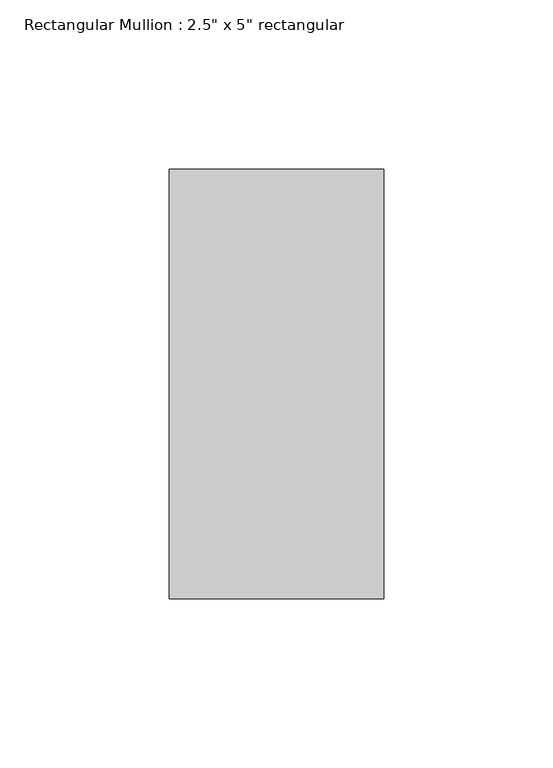
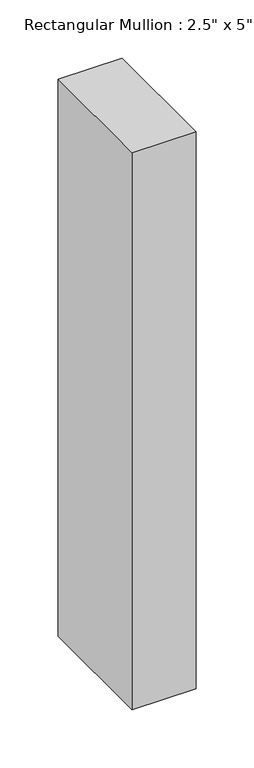
"""IFC4 building model written with IfcOpenShell, lengths in millimetres: member geometry."""

from ifc_helpers import new_model, si_unit, frame, origin, place, context, project, spatial, polyline, outline, extrude, source, transform, mapped, element, save


def member_39111128(model_context):
    return source(origin(), model_context, "Body", "SweptSolid", [
        extrude(outline(polyline([(0.0, 63.5), (0.0, -63.5), (-63.5, -63.5), (-63.5, 63.5), (0.0, 63.5)])), frame((0.0, 0.0, -584.2173759), z_axis=(0.0, 0.0, 1.0), x_axis=(1.0, 0.0, 0.0)), (0.0, 0.0, 1.0), 584.2173759),
    ])


if __name__ == "__main__":
    model = new_model("IFC4")
    model_context = context("Model", 3, world=origin())
    ifc_project = project(units=[si_unit("LENGTHUNIT", "METRE", prefix="MILLI")], contexts=[model_context])
    site = spatial("IfcSite", under=ifc_project)
    building = spatial("IfcBuilding", under=site)
    placement = place(None, origin())
    member_shape = member_39111128(model_context)
    element("IfcMember", 1, ObjectType="Rectangular Mullion : 2.5\" x 5\" rectangular", at=placement, inside=building, context=model_context, shape_type="MappedRepresentation", body=[
        mapped(member_shape, transform((0.0, 0.0, 0.0), x_axis=(1.0, 0.0, 0.0), y_axis=(0.0, 1.0, 0.0), z_axis=(0.0, 0.0, 1.0))),
    ])
    save(model, "model.ifc")

# Revit data of these elements
# Type "Rectangular Mullion : 2.5\" x 5\" rectangular"
#   built-in parameter 1007304 = 0.416667 (stored number, unit not read)
#   built-in parameter 1007301 = 0.104167 (stored number, unit not read)
#   built-in parameter 1007300 = 0.104167 (stored number, unit not read)
# Element 1 (IfcMember, "Rectangular Mullion : 2.5\" x 5\" rectangular")
#   Materials on its faces: "Aluminum"
# Materials
#   "Aluminum": class "Metal", colour RGB 247 247 247, transparency 0, Description = "Aluminum 6061", Cost = 0
